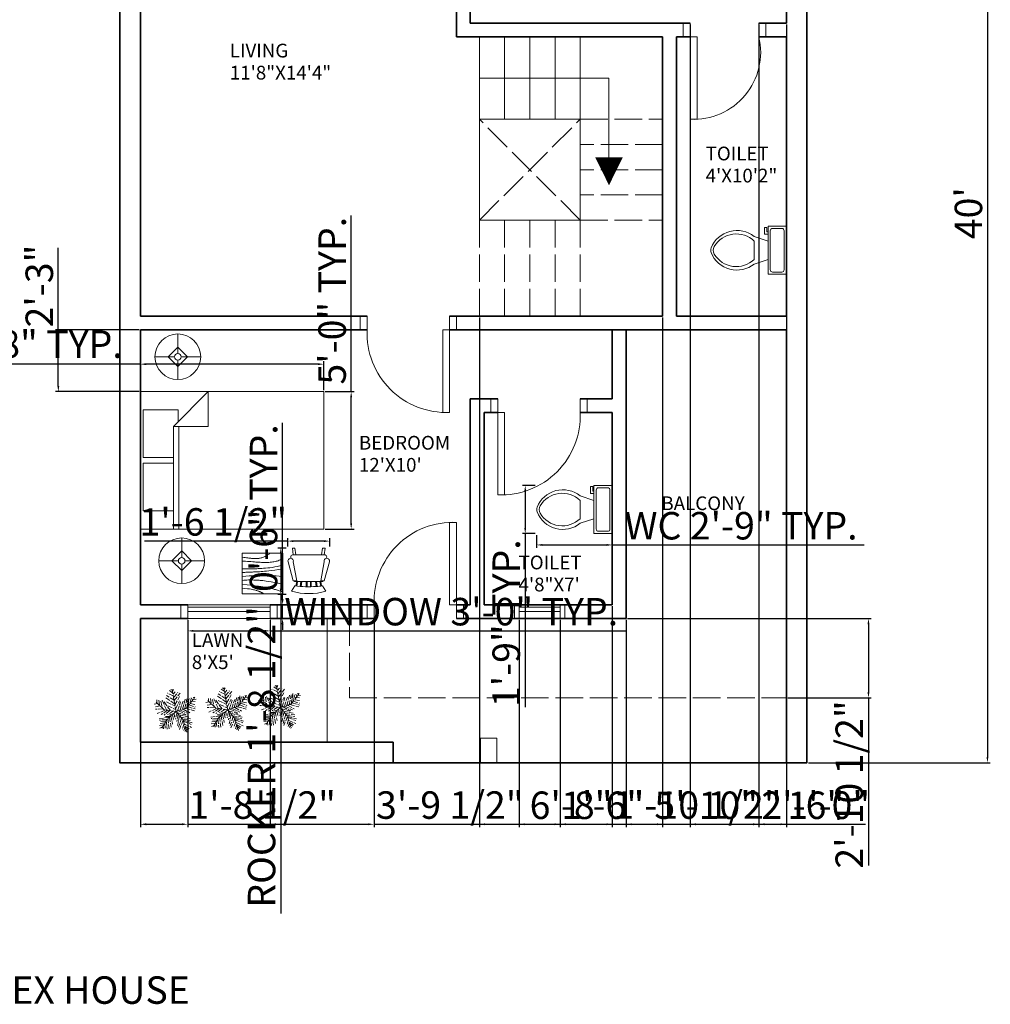
# Model space of a CAD drawing. Units: inches. Extents: x 2446 to 3341, y 462 to 1195.
# Tile 5 of 6: x 2884 to 3308, y 462 to 892. Entities that reach past the tile are written whole.
import ezdxf

# ---------------------------------------------------------------- set-up
doc = ezdxf.new("R2010")
doc.units = ezdxf.units.IN
doc.linetypes.add('ACAD_ISO02W100', pattern=[15, 12, -3])
for name, color, linetype, lineweight in [('A-ANNO-DIMS', 2, 'Continuous', 18), ('A-ANNO-TEXT', 7, 'Continuous', 25), ('A-AREA-IDEN', 7, 'Continuous', 18), ('A-DOOR', 4, 'Continuous', 18), ('A-FLOR-FIXT', 9, 'Continuous', 18), ('A-FLOR-HIDN', 8, 'ACAD_ISO02W100', 18), ('A-FLOR-STRS', 7, 'Continuous', 18), ('A-FLOR-STRS-HIDN', 8, 'ACAD_ISO02W100', 18), ('A-FURN', 8, 'Continuous', 18), ('A-GLAZ', 4, 'Continuous', 18), ('A-WALL', 7, 'Continuous', 35), ('C-PROP', 7, 'Continuous', 35), ('L-PLNT', 3, 'Continuous', 18), ('L-PLNT-BELO', 3, 'ACAD_ISO02W100', 13)]:
    doc.layers.add(name, color=color, linetype=linetype, lineweight=lineweight)
doc.styles.get("Standard").update_dxf_attribs({"font": 'arial.ttf'})
doc.dimstyles.new('ISO-25', dxfattribs={"dimtxt": 12, "dimasz": 2.5, "dimexe": 1.25, "dimexo": 0.625, "dimtad": 1, "dimdec": 1, "dimlunit": 3, "dimtxsty": 'Standard', "dimcen": 2.5, "dimadec": 0, "dimazin": 0, "dimtfac": 1, "dimtdec": 1, "dimtmove": 0, "dimatfit": 3, "dimfxl": 1, "dimarcsym": 0})

# ---------------------------------------------------------------- blocks, each defined once
blk = doc.blocks.new('Toilet - top')
for p, q in [((9.5, -6), (9.5, -2)), ((-10, -8.5), (-8, -8.5)), ((-10, -9.5), (-10, -8.5)), ((-8, -8.5), (-8, -8)), ((-7, -8), (-7, -9.5)), ((-4, -8), (-6, -14)), ((4, -8), (6, -14)), ((-7, -9.5), (-10, -9.5)), ((4, -14), (-4, -14))]:
    blk.add_line(p, q)
blk.add_lwpolyline([(10.5, -8), (10.5, 0), (-10.5, 0), (-10.5, -8)], close=True)
for points in [[(-9.5, -2), (-9.5, -6)], [(8.5, -1), (-8.5, -1)], [(-8.5, -7), (8.5, -7)]]:
    blk.add_lwpolyline(points)
for centre, radius, start, end in [((-8.62, -1.88), 0.884, 81.8699, 188.1301), ((8.62, -1.88), 0.884, 351.8699, 98.1301), ((-8.62, -6.12), 0.884, 171.8699, 278.1301), ((8.62, -6.12), 0.884, 261.8699, 8.1301), ((3.52, -21.58), 12.17, 141.4691, 247.9714), ((4.2, -21.82), 11.33, 136.3677, 238.9468), ((-3.52, -21.58), 12.17, 292.0284, 38.5307), ((-4.2, -21.82), 11.33, 301.053, 43.6321), ((0, -27.88), 4, 245.7318, 294.2682), ((0, -29), 4, 254.8605, 285.1395)]:
    blk.add_arc(centre, radius, start, end)
blk = doc.blocks.new('Bed - Queen')
for p, q in [((0, -80.00003), (0, 0)), ((0, 0), (59.99999, 0)), ((59.99999, 0), (59.99999, -80.00003)), ((7.99999, -1.2), (28.79998, -1.2)), ((7.99999, -14.4), (7.99999, -1.2)), ((28.79998, -1.2), (28.79998, -14.4)), ((31.19999, -1.2), (51.99999, -1.2)), ((31.19999, -14.4), (31.19999, -1.2)), ((51.99999, -1.2), (51.99999, -16.4)), ((0, -14.4), (44.8, -14.4)), ((44.8, -16.8), (0, -16.8)), ((59.99999, -29.6), (44.8, -14.4)), ((44.8, -14.4), (44.8, -29.6)), ((51.99999, -16.4), (46.79936, -16.4)), ((44.8, -29.6), (59.99999, -29.6)), ((59.99999, -80.00003), (0, -80.00003))]:
    blk.add_line(p, q)
blk = doc.blocks.new('Lamp - Table')
for p, q in [((0, 7), (0, 1)), ((-1, 0), (-7, 0)), ((0, 3), (-3, 0)), ((-3, 0), (0, -3)), ((3, 0), (0, 3)), ((0, -3), (3, 0)), ((1, 0), (7, 0)), ((0, -1), (0, -7))]:
    blk.add_line(p, q)
for radius in [7, 1]:
    blk.add_circle((0, 0), radius)
blk = doc.blocks.new('Chair - Rocking')
for p, q in [((-8, -4.5), (-10, -1.5)), ((-7.5, -4.5), (-7, -7)), ((-6.5, -7), (-7.02225, -4.43)), ((-4.5, -7), (-4.96674, -4.19951)), ((-4, -7), (-4.40532, -4.16272)), ((-1.5, -4.05012), (-1.5, -7)), ((-1, -7), (-1, -4.05012)), ((1, -7), (1, -4.04655)), ((1.5, -4.05012), (1.5, -7)), ((4, -7), (4.40187, -4.18694)), ((4.5, -7), (4.96761, -4.19437)), ((6.5, -7), (7, -4.4057)), ((7.5, -4.5), (7, -7)), ((8, -4.5), (10, -1.5)), ((-9, -7.5), (-12, -18.49999)), ((-7, -7.5), (-9, -7.5)), ((-9, -18.49999), (-7, -7.5)), ((-8.23428, -6.99939), (-8.3093, -7.47958)), ((-8.23041, -7), (8.23915, -7)), ((7, -7.5), (9, -7.5)), ((9, -18.49999), (7, -7.5)), ((8.31071, -7.48854), (8.23449, -7.00073)), ((9, -7.5), (12, -18.49999)), ((-10.36644, -20.64523), (-10.5, -21.49999)), ((-9, -22.49999), (-9.5, -26.49999)), ((0, -22.49999), (-9.5, -22.49999)), ((-8, -26.49999), (-7.5, -22.49999)), ((0, -22.49999), (9.5, -22.49999)), ((8, -26.49999), (7.5, -22.49999)), ((9, -22.49999), (9.5, -26.49999)), ((10.5, -21.49999), (10.3575, -20.58798)), ((-9.5, -26.49999), (-8, -26.49999)), ((9.5, -26.49999), (8, -26.49999))]:
    blk.add_line(p, q)
for centre, radius, start, end in [((0, -34.08333), 34.08333, 72.93847, 107.0615), ((0, -68.25004), 64.25, 93.92211, 97.15267), ((0, -68.25004), 64.25, 82.84733, 93.92211), ((-10.5, -18.99999), 1.58114, 161.5651, 18.43495), ((-9.5, -21.49999), 1, 180, 270), ((10.5, -18.99999), 1.58114, 161.5651, 18.43495), ((9.5, -21.49999), 1, 270, 0)]:
    blk.add_arc(centre, radius, start, end)
blk = doc.blocks.new('Table - Square Woodgrain 42 x 42 in.')
blk.add_line((0, -42), (42, -42))
for points in [[(0, -4), (1.704, -4.2172), (3.2358, -4.4188), (4.615, -4.604), (5.8615, -4.7721), (6.9951, -4.9224), (8.0357, -5.0541), (9.0031, -5.1667), (9.9171, -5.2594), (10.7951, -5.3316), (11.6445, -5.3836), (12.4702, -5.4157), (13.277, -5.4283), (14.0698, -5.4217), (14.8535, -5.3964), (15.6331, -5.3526), (16.4133, -5.2908), (17.1986, -5.2103), (17.9913, -5.1062), (18.793, -4.9727), (19.6056, -4.8038), (20.4307, -4.5937), (21.2701, -4.3365), (22.1256, -4.0262), (22.9989, -3.6571), (23.888, -3.2272), (24.7756, -2.7516), (25.6408, -2.2491), (26.4624, -1.7387), (27.2195, -1.2395), (27.891, -0.7703), (28.456, -0.3501), (28.8934, 0.002)], [(0, -42), (0, 0), (42, 0), (42, -42)], [(0, -8), (1.8203, -8.1001), (3.6741, -8.2149), (5.5411, -8.3408), (7.4011, -8.4741), (9.2339, -8.6112), (11.0193, -8.7484), (12.7371, -8.8821), (14.3671, -9.0086), (15.8954, -9.1246), (17.3337, -9.2278), (18.6997, -9.3159), (20.0116, -9.387), (21.2871, -9.4389), (22.5442, -9.4696), (23.8008, -9.477), (25.0749, -9.459), (26.3791, -9.4137), (27.7049, -9.3403), (29.0383, -9.2382), (30.3655, -9.1068), (31.6728, -8.9455), (32.9461, -8.7535), (34.1717, -8.5304), (35.3358, -8.2756), (36.4268, -7.9863), (37.443, -7.6521), (38.3849, -7.2603), (39.253, -6.7986), (40.048, -6.2542), (40.7705, -5.6147), (41.421, -4.8674), (42, -4)], [(42, -12), (39.1784, -12.8621), (36.4519, -13.5654), (33.8246, -14.1294), (31.3004, -14.5731), (28.8832, -14.9161), (26.577, -15.1775), (24.3858, -15.3768), (22.3136, -15.5332), (20.3622, -15.6632), (18.5254, -15.7718), (16.7947, -15.8612), (15.1618, -15.9338), (13.6183, -15.9916), (12.1558, -16.0369), (10.7659, -16.0718), (9.4403, -16.0987), (8.1703, -16.1191), (6.9461, -16.1325), (5.7577, -16.1377), (4.595, -16.1335), (3.4479, -16.1188), (2.3064, -16.0924), (1.1604, -16.0532), (0, -16)], [(42, -16), (37.6529, -16.7365), (33.8802, -17.329), (30.6179, -17.7961), (27.8015, -18.1561), (25.3668, -18.4275), (23.2497, -18.6288), (21.3859, -18.7785), (19.7111, -18.8949), (18.1693, -18.9939), (16.7375, -19.0795), (15.401, -19.1534), (14.1449, -19.217), (12.9544, -19.2717), (11.8148, -19.3191), (10.7113, -19.3606), (9.6291, -19.3976), (8.5534, -19.4323), (7.47, -19.4689), (6.3643, -19.5122), (5.222, -19.5672), (4.0288, -19.6386), (2.7703, -19.7313), (1.4321, -19.8501), (0, -20)], [(0, -24), (3.9243, -23.6805), (7.4766, -23.4138), (10.6891, -23.1954), (13.5943, -23.0205), (16.2247, -22.8847), (18.6125, -22.7832), (20.7903, -22.7116), (22.7903, -22.6651), (24.6563, -22.642), (26.4764, -22.6507), (28.35, -22.7024), (30.3766, -22.8084), (32.6555, -22.98), (35.2861, -23.2283), (38.3678, -23.5645), (42, -24)], [(42, -32), (37.392, -31.017), (33.4585, -30.2231), (30.1291, -29.5949), (27.3334, -29.109), (25.0009, -28.742), (23.0612, -28.4707), (21.4439, -28.2716), (20.0786, -28.1215), (18.8998, -28.0002), (17.8609, -27.9014), (16.9206, -27.8219), (16.0371, -27.7588), (15.1691, -27.709), (14.2748, -27.6693), (13.3128, -27.6368), (12.2415, -27.6083), (11.0295, -27.5824), (9.6867, -27.5643), (8.233, -27.5608), (6.6884, -27.5787), (5.0728, -27.6248), (3.4062, -27.7058), (1.7086, -27.8286), (0, -28)], [(0, -32), (5.4026, -32.5358), (9.9494, -33.019), (13.7424, -33.4553), (16.8834, -33.8505), (19.4743, -34.2106), (21.6171, -34.5413), (23.4136, -34.8486), (24.9657, -35.1382), (26.3614, -35.4156), (27.6332, -35.6841), (28.7995, -35.9467), (29.8788, -36.2064), (30.8897, -36.4661), (31.8507, -36.7288), (32.7802, -36.9973), (33.6968, -37.2747), (34.6175, -37.5635), (35.5531, -37.8651), (36.5128, -38.1805), (37.506, -38.5108), (38.5421, -38.8568), (39.6302, -39.2197), (40.7797, -39.6004), (42, -40)], [(0, -36), (3.0098, -36.2857), (5.5354, -36.5643), (7.6368, -36.8359), (9.374, -37.1009), (10.807, -37.3597), (11.9957, -37.6126), (13.0002, -37.8599), (13.8804, -38.102), (14.6874, -38.3393), (15.4365, -38.5729), (16.1338, -38.8041), (16.7858, -39.0341), (17.3987, -39.264), (17.9787, -39.4952), (18.5322, -39.7288), (19.0655, -39.9662), (19.5832, -40.2081), (20.0842, -40.4544), (20.5657, -40.7046), (21.0249, -40.9581), (21.459, -41.2144), (21.8653, -41.4731), (22.2409, -41.7335), (22.5831, -41.9951)]]:
    blk.add_lwpolyline(points)
blk = doc.blocks.new('*U16')
for p, q in [((-8.737, 47.138), (-17.069, 52.711)), ((-10.186, 53.64), (-13.084, 55.962)), ((0, 0), (-10.5, 57)), ((-9.099, 51.782), (-6.563, 55.962)), ((-31.5, 4.5), (-52.5, 25.5)), ((-48.585, 21.131), (-49.309, 29.026)), ((-43.513, 28.561), (-42.427, 15.558)), ((-38.442, 26.239), (-34.819, 7.663)), ((-35.544, 28.097), (-24.314, 3.947)), ((-14.533, 2.09), (-30.834, 25.31)), ((-3.665, 19.273), (-27.574, 35.527)), ((-5.114, 28.097), (-24.676, 40.636)), ((-7.288, 39.707), (-21.778, 46.673)), ((-7.65, 43.423), (-2.578, 49.46)), ((-5.839, 35.992), (4.667, 48.067)), ((-5.114, 27.632), (10.463, 46.673)), ((-2.941, 16.486), (8.652, 37.85)), ((-1.129, 6.734), (9.014, 26.704)), ((10.101, 3.483), (17.708, 26.239)), ((16.259, 5.805), (23.142, 31.348)), ((22.055, 7.198), (27.489, 32.277)), ((27, 9), (48, 36)), ((27.127, 9.056), (31.112, 35.992)), ((31.836, 30.883), (32.561, 16.486)), ((35.096, 32.741), (37.27, 22.524)), ((38.719, 34.134), (41.979, 28.561)), ((40.53, 25.775), (48.862, 24.846)), ((43.791, 29.954), (51.036, 30.883)), ((44.153, 36.456), (45.239, 32.741)), ((-47.498, 19.737), (-55.83, 18.344)), ((-40.615, 13.7), (-55.105, 10.913)), ((-33.37, 6.269), (-52.207, 5.34)), ((-28.299, 3.483), (-47.86, -5.805)), ((-21.416, 3.018), (-38.079, -8.128)), ((0, 0), (-31.5, 4.5)), ((-15.982, 2.09), (-30.11, -9.521)), ((-24.314, 23.917), (-2.941, 13.7)), ((0, 0), (-22.5, -19.5)), ((-6.563, 1.161), (-21.416, -8.128)), ((-20.691, 13.7), (-1.129, 4.876)), ((0, 0), (27, 9)), ((0, 0), (18, -22.5)), ((3.942, 1.625), (11.187, 24.381)), ((6.478, 1.625), (26.04, -8.592)), ((11.187, 3.483), (30.749, -5.805)), ((18.07, 5.805), (35.096, -3.483)), ((24.229, 7.663), (46.688, 1.625)), ((29.662, 12.307), (48.137, 6.269)), ((33.285, 16.486), (48.862, 10.913)), ((36.183, 19.737), (48.137, 17.88)), ((-17.431, -15.094), (-42.789, -18.809)), ((-24.314, -21.596), (-42.427, -22.06)), ((-22.5, -19.5), (-37.5, -45)), ((-15.257, -12.772), (-30.11, -12.772)), ((-25.038, -23.918), (-22.865, -45.281)), ((-20.691, -18.345), (-17.793, -44.352)), ((-6.563, -5.805), (-19.967, -9.985)), ((-17.069, -15.094), (-12.721, -40.172)), ((-13.446, -11.378), (-8.737, -32.741)), ((-9.461, -8.592), (-6.201, -23.453)), ((-4.752, -3.483), (-3.665, -14.629)), ((2.493, -3.019), (-1.491, -20.202)), ((1.769, -2.555), (24.229, -9.521)), ((5.029, -6.27), (2.131, -25.775)), ((9.014, -11.378), (3.58, -35.992)), ((14.085, -16.951), (6.478, -40.172)), ((7.565, -9.056), (32.198, -14.629)), ((18.07, -22.524), (8.289, -45.745)), ((12.274, -15.094), (36.907, -18.809)), ((16.259, -19.738), (36.183, -22.989)), ((18, -22.5), (27, -52.5)), ((18.433, -22.524), (40.53, -29.026)), ((-28.299, -29.026), (-42.789, -31.348)), ((-30.834, -34.135), (-42.427, -35.528)), ((-34.457, -39.708), (-40.978, -42.494)), ((-26.849, -26.24), (-40.253, -25.775)), ((-32.646, -36.921), (-31.921, -44.352)), ((-29.023, -30.884), (-27.936, -43.887)), ((20.244, -30.419), (15.897, -44.816)), ((19.157, -25.311), (38.719, -33.206)), ((22.78, -37.85), (19.519, -48.532)), ((21.331, -32.741), (39.081, -40.636)), ((22.78, -38.314), (34.372, -44.816)), ((24.591, -45.745), (23.142, -50.854)), ((24.591, -43.423), (30.749, -47.603)), ((26.764, -49.925), (28.213, -50.854))]:
    blk.add_line(p, q)
blk = doc.blocks.new('*D20')
at = {"layer": 'A-ANNO-DIMS', "color": 0, "lineweight": -2, "transparency": 16777216}
for p, q in [((3228.82, 1047.51), (3308.24, 1047.51)), ((3306.99, 1045.01), (3306.99, 570.01)), ((3228.82, 567.51), (3308.24, 567.51))]:
    blk.add_line(p, q, dxfattribs=at)
at = {"layer": 'A-ANNO-DIMS', "color": 0, "transparency": 16777216}
for points in [[(3306.57, 1045.01), (3307.4, 1045.01), (3306.99, 1047.51)], [(3306.57, 570.01), (3307.4, 570.01), (3306.99, 567.51)]]:
    blk.add_solid(points, dxfattribs=at)
at = {"layer": 'Defpoints', "color": 0, "transparency": 16777216}
for p in [(3228.19, 1047.51), (3228.19, 567.51), (3306.99, 567.51)]:
    blk.add_point(p, dxfattribs=at)
at = {"layer": 'A-ANNO-DIMS', "color": 0, "transparency": 16777216, "insert": (3300.24, 807.51), "char_height": 12, "attachment_point": 5, "rotation": 90}
blk.add_mtext("40'", dxfattribs=at)
blk = doc.blocks.new('DOOR-SWING-36IN')
for p, q in [((6, 42), (0, 42)), ((6, 39), (0, 39)), ((6, 3), (0, 3)), ((6, 0), (0, 0))]:
    blk.add_line(p, q)
blk.add_lwpolyline([(6, 3), (42, 3), (42, 6), (6, 6)], close=True)
blk.add_arc((7.5, 4.5), 34.53, 357.5104, 92.4896)
blk = doc.blocks.new('WIN-36IN')
for p, q in [((0, 6), (0, 0)), ((0, 5), (36, 5)), ((36, 0), (36, 6)), ((0, 3), (36, 3))]:
    blk.add_line(p, q)
blk = doc.blocks.new('*D29')
at = {"layer": 'A-ANNO-DIMS', "color": 0, "lineweight": -2, "transparency": 16777216}
for p, q in [((2937.19, 741.58), (2756.92, 741.58)), ((2937.19, 730.2), (2937.19, 742.83)), ((3014.69, 741.58), (2939.69, 741.58)), ((3017.19, 730.2), (3017.19, 742.83))]:
    blk.add_line(p, q, dxfattribs=at)
at = {"layer": 'A-ANNO-DIMS', "color": 0, "transparency": 16777216}
for points in [[(2939.69, 742), (2939.69, 741.16), (2937.19, 741.58)], [(3014.69, 742), (3014.69, 741.16), (3017.19, 741.58)]]:
    blk.add_solid(points, dxfattribs=at)
at = {"layer": 'Defpoints', "color": 0, "transparency": 16777216}
for p in [(2937.19, 741.58), (2937.19, 729.58), (3017.19, 729.58)]:
    blk.add_point(p, dxfattribs=at)
at = {"layer": 'A-ANNO-DIMS', "color": 0, "transparency": 16777216, "insert": (2845.81, 748.78), "char_height": 12, "attachment_point": 5}
blk.add_mtext('QUEEN BED 6\'-8" TYP.', dxfattribs=at)
blk = doc.blocks.new('*D30')
at = {"layer": 'A-ANNO-DIMS', "color": 0, "lineweight": -2, "transparency": 16777216}
for p, q in [((3029.19, 729.58), (3029.19, 806.47)), ((3017.82, 729.58), (3030.44, 729.58)), ((3029.19, 672.08), (3029.19, 727.08)), ((3017.82, 669.58), (3030.44, 669.58))]:
    blk.add_line(p, q, dxfattribs=at)
at = {"layer": 'A-ANNO-DIMS', "color": 0, "transparency": 16777216}
for points in [[(3028.78, 727.08), (3029.61, 727.08), (3029.19, 729.58)], [(3028.78, 672.08), (3029.61, 672.08), (3029.19, 669.58)]]:
    blk.add_solid(points, dxfattribs=at)
at = {"layer": 'Defpoints', "color": 0, "transparency": 16777216}
for p in [(3017.19, 729.58), (3029.19, 729.58), (3017.19, 669.58)]:
    blk.add_point(p, dxfattribs=at)
at = {"layer": 'A-ANNO-DIMS', "color": 0, "transparency": 16777216, "insert": (3022.44, 769.28), "char_height": 12, "attachment_point": 5, "rotation": 90}
blk.add_mtext('5\'-0" TYP.', dxfattribs=at)
blk = doc.blocks.new('*D31')
at = {"layer": 'A-ANNO-DIMS', "color": 0, "lineweight": -2, "transparency": 16777216}
for p, q in [((3110.15, 666.97), (3110.15, 661.39)), ((3143.19, 666.97), (3143.19, 661.39)), ((3112.65, 662.64), (3140.69, 662.64)), ((3143.19, 662.64), (3253.17, 662.64))]:
    blk.add_line(p, q, dxfattribs=at)
at = {"layer": 'A-ANNO-DIMS', "color": 0, "transparency": 16777216}
for points in [[(3112.65, 663.05), (3112.65, 662.22), (3110.15, 662.64)], [(3140.69, 663.05), (3140.69, 662.22), (3143.19, 662.64)]]:
    blk.add_solid(points, dxfattribs=at)
at = {"layer": 'Defpoints', "color": 0, "transparency": 16777216}
for p in [(3110.15, 667.59), (3143.19, 667.59), (3143.19, 662.64)]:
    blk.add_point(p, dxfattribs=at)
at = {"layer": 'A-ANNO-DIMS', "color": 0, "transparency": 16777216, "insert": (3199.43, 669.47), "char_height": 12, "attachment_point": 5}
blk.add_mtext('WC 2\'-9" TYP.', dxfattribs=at)
blk = doc.blocks.new('*D32')
at = {"layer": 'A-ANNO-DIMS', "color": 0, "lineweight": -2, "transparency": 16777216}
for p, q in [((3109.52, 688.59), (3103.94, 688.59)), ((3105.19, 686.09), (3105.19, 670.09)), ((3109.52, 667.59), (3103.94, 667.59)), ((3105.19, 667.59), (3105.19, 591.83))]:
    blk.add_line(p, q, dxfattribs=at)
at = {"layer": 'A-ANNO-DIMS', "color": 0, "transparency": 16777216}
for points in [[(3104.77, 686.09), (3105.61, 686.09), (3105.19, 688.59)], [(3104.77, 670.09), (3105.61, 670.09), (3105.19, 667.59)]]:
    blk.add_solid(points, dxfattribs=at)
at = {"layer": 'Defpoints', "color": 0, "transparency": 16777216}
for p in [(3110.15, 688.59), (3105.19, 667.59), (3110.15, 667.59)]:
    blk.add_point(p, dxfattribs=at)
at = {"layer": 'A-ANNO-DIMS', "color": 0, "transparency": 16777216, "insert": (3098.44, 628.46), "char_height": 12, "attachment_point": 5, "rotation": 90}
blk.add_mtext('1\'-9" TYP.', dxfattribs=at)
blk = doc.blocks.new('*D35')
at = {"layer": 'A-ANNO-DIMS', "color": 0, "lineweight": -2, "transparency": 16777216}
for p, q in [((3000.87, 661.27), (2997.2, 661.27)), ((2998.45, 658.77), (2998.45, 643.5)), ((3000.87, 641), (2997.2, 641)), ((2998.45, 641), (2998.45, 501.63))]:
    blk.add_line(p, q, dxfattribs=at)
at = {"layer": 'A-ANNO-DIMS', "color": 0, "transparency": 16777216}
for points in [[(2998.03, 658.77), (2998.87, 658.77), (2998.45, 661.27)], [(2998.03, 643.5), (2998.87, 643.5), (2998.45, 641)]]:
    blk.add_solid(points, dxfattribs=at)
at = {"layer": 'Defpoints', "color": 0, "transparency": 16777216}
for p in [(3001.49, 661.27), (2998.45, 641), (3001.49, 641)]:
    blk.add_point(p, dxfattribs=at)
at = {"layer": 'A-ANNO-DIMS', "color": 0, "transparency": 16777216, "insert": (2991.62, 570.06), "char_height": 12, "attachment_point": 5, "rotation": 90}
blk.add_mtext('ROCKER 1\'-8 1/2"', dxfattribs=at)
blk = doc.blocks.new('*D36')
at = {"layer": 'A-ANNO-DIMS', "color": 0, "lineweight": -2, "transparency": 16777216}
for p, q in [((3001.49, 664.31), (2939.01, 664.31)), ((3001.49, 661.89), (3001.49, 665.56)), ((3017.33, 664.31), (3003.99, 664.31)), ((3019.83, 661.89), (3019.83, 665.56))]:
    blk.add_line(p, q, dxfattribs=at)
at = {"layer": 'A-ANNO-DIMS', "color": 0, "transparency": 16777216}
for points in [[(3003.99, 664.72), (3003.99, 663.89), (3001.49, 664.31)], [(3017.33, 664.72), (3017.33, 663.89), (3019.83, 664.31)]]:
    blk.add_solid(points, dxfattribs=at)
at = {"layer": 'Defpoints', "color": 0, "transparency": 16777216}
for p in [(3001.49, 664.31), (3001.49, 661.27), (3019.83, 661.27)]:
    blk.add_point(p, dxfattribs=at)
at = {"layer": 'A-ANNO-DIMS', "color": 0, "transparency": 16777216, "insert": (2969, 671.14), "char_height": 12, "attachment_point": 5}
blk.add_mtext('1\'-6 1/2"', dxfattribs=at)
blk = doc.blocks.new('*D49')
at = {"layer": 'A-ANNO-DIMS', "color": 0, "lineweight": -2, "transparency": 16777216}
for p, q in [((2957.84, 629.89), (2957.84, 623.86)), ((2993.84, 629.89), (2993.84, 623.86)), ((2960.34, 625.11), (2991.34, 625.11)), ((2993.84, 625.11), (3149.44, 625.11))]:
    blk.add_line(p, q, dxfattribs=at)
at = {"layer": 'A-ANNO-DIMS', "color": 0, "transparency": 16777216}
for points in [[(2960.34, 625.53), (2960.34, 624.69), (2957.84, 625.11)], [(2991.34, 625.53), (2991.34, 624.69), (2993.84, 625.11)]]:
    blk.add_solid(points, dxfattribs=at)
at = {"layer": 'Defpoints', "color": 0, "transparency": 16777216}
for p in [(2957.84, 630.51), (2993.84, 630.51), (2993.84, 625.11)]:
    blk.add_point(p, dxfattribs=at)
at = {"layer": 'A-ANNO-DIMS', "color": 0, "transparency": 16777216, "insert": (3072.89, 631.95), "char_height": 12, "attachment_point": 5}
blk.add_mtext('WINDOW 3\'-0" TYP.', dxfattribs=at)
blk = doc.blocks.new('*D50')
at = {"layer": 'A-ANNO-DIMS', "color": 0, "lineweight": -2, "transparency": 16777216}
for p, q in [((2999.24, 639.01), (2999.24, 715.91)), ((2994.47, 636.51), (3000.49, 636.51)), ((2999.24, 630.51), (2999.24, 636.51)), ((2994.47, 630.51), (3000.49, 630.51)), ((2999.24, 628.01), (2999.24, 625.51))]:
    blk.add_line(p, q, dxfattribs=at)
at = {"layer": 'A-ANNO-DIMS', "color": 0, "transparency": 16777216}
for points in [[(2998.83, 639.01), (2999.66, 639.01), (2999.24, 636.51)], [(2998.83, 628.01), (2999.66, 628.01), (2999.24, 630.51)]]:
    blk.add_solid(points, dxfattribs=at)
at = {"layer": 'Defpoints', "color": 0, "transparency": 16777216}
for p in [(2993.84, 636.51), (2999.24, 636.51), (2993.84, 630.51)]:
    blk.add_point(p, dxfattribs=at)
at = {"layer": 'A-ANNO-DIMS', "color": 0, "transparency": 16777216, "insert": (2992.49, 678.71), "char_height": 12, "attachment_point": 5, "rotation": 90}
blk.add_mtext('0\'-6" TYP.', dxfattribs=at)
blk = doc.blocks.new('*D61')
at = {"layer": 'A-ANNO-DIMS', "color": 0, "lineweight": -2, "transparency": 16777216}
for p, q in [((3085.19, 761.89), (3085.19, 539.41)), ((3165.19, 761.89), (3165.19, 539.41)), ((3087.69, 540.66), (3162.69, 540.66))]:
    blk.add_line(p, q, dxfattribs=at)
at = {"layer": 'A-ANNO-DIMS', "color": 0, "transparency": 16777216}
for points in [[(3087.69, 541.08), (3087.69, 540.24), (3085.19, 540.66)], [(3162.69, 541.08), (3162.69, 540.24), (3165.19, 540.66)]]:
    blk.add_solid(points, dxfattribs=at)
at = {"layer": 'Defpoints', "color": 0, "transparency": 16777216}
for p in [(3085.19, 762.51), (3165.19, 762.51), (3165.19, 540.66)]:
    blk.add_point(p, dxfattribs=at)
at = {"layer": 'A-ANNO-DIMS', "color": 0, "transparency": 16777216, "insert": (3125.19, 547.41), "char_height": 12, "attachment_point": 5}
blk.add_mtext('6\'-8"', dxfattribs=at)
blk = doc.blocks.new('*D65')
at = {"layer": 'A-ANNO-DIMS', "color": 0, "lineweight": -2, "transparency": 16777216}
for p, q in [((3149.19, 629.89), (3149.19, 539.41)), ((3219.19, 595.22), (3219.19, 539.41)), ((3151.69, 540.66), (3216.69, 540.66))]:
    blk.add_line(p, q, dxfattribs=at)
at = {"layer": 'A-ANNO-DIMS', "color": 0, "transparency": 16777216}
for points in [[(3151.69, 541.08), (3151.69, 540.24), (3149.19, 540.66)], [(3216.69, 541.08), (3216.69, 540.24), (3219.19, 540.66)]]:
    blk.add_solid(points, dxfattribs=at)
at = {"layer": 'Defpoints', "color": 0, "transparency": 16777216}
for p in [(3149.19, 630.51), (3219.19, 595.85), (3219.19, 540.66)]:
    blk.add_point(p, dxfattribs=at)
at = {"layer": 'A-ANNO-DIMS', "color": 0, "transparency": 16777216, "insert": (3184.19, 547.41), "char_height": 12, "attachment_point": 5}
blk.add_mtext('5\'-10"', dxfattribs=at)
blk = doc.blocks.new('*D66')
at = {"layer": 'A-ANNO-DIMS', "color": 0, "lineweight": -2, "transparency": 16777216}
for p, q in [((3149.82, 630.51), (3256.29, 630.51)), ((3255.04, 628.01), (3255.04, 598.35)), ((3219.82, 595.85), (3256.29, 595.85)), ((3255.04, 595.85), (3255.04, 522.71))]:
    blk.add_line(p, q, dxfattribs=at)
at = {"layer": 'A-ANNO-DIMS', "color": 0, "transparency": 16777216}
for points in [[(3254.63, 628.01), (3255.46, 628.01), (3255.04, 630.51)], [(3254.63, 598.35), (3255.46, 598.35), (3255.04, 595.85)]]:
    blk.add_solid(points, dxfattribs=at)
at = {"layer": 'Defpoints', "color": 0, "transparency": 16777216}
for p in [(3149.19, 630.51), (3219.19, 595.85), (3255.04, 595.85)]:
    blk.add_point(p, dxfattribs=at)
at = {"layer": 'A-ANNO-DIMS', "color": 0, "transparency": 16777216, "insert": (3248.21, 558.03), "char_height": 12, "attachment_point": 5, "rotation": 90}
blk.add_mtext('2\'-10 1/2"', dxfattribs=at)
blk = doc.blocks.new('*D69')
at = {"layer": 'A-ANNO-DIMS', "color": 0, "lineweight": -2, "transparency": 16777216}
for p, q in [((3102.48, 629.89), (3102.48, 539.41)), ((3120.48, 629.89), (3120.48, 539.41)), ((3104.98, 540.66), (3117.98, 540.66)), ((3120.48, 540.66), (3155, 540.66))]:
    blk.add_line(p, q, dxfattribs=at)
at = {"layer": 'A-ANNO-DIMS', "color": 0, "transparency": 16777216}
for points in [[(3104.98, 541.08), (3104.98, 540.24), (3102.48, 540.66)], [(3117.98, 541.08), (3117.98, 540.24), (3120.48, 540.66)]]:
    blk.add_solid(points, dxfattribs=at)
at = {"layer": 'Defpoints', "color": 0, "transparency": 16777216}
for p in [(3102.48, 630.51), (3120.48, 630.51), (3120.48, 540.66)]:
    blk.add_point(p, dxfattribs=at)
at = {"layer": 'A-ANNO-DIMS', "color": 0, "transparency": 16777216, "insert": (3138.99, 547.41), "char_height": 12, "attachment_point": 5}
blk.add_mtext('1\'-6"', dxfattribs=at)
blk = doc.blocks.new('*D70')
at = {"layer": 'A-ANNO-DIMS', "color": 0, "lineweight": -2, "transparency": 16777216}
for p, q in [((3143.19, 635.89), (3143.19, 539.41)), ((3120.48, 629.89), (3120.48, 539.41)), ((3122.98, 540.66), (3140.69, 540.66)), ((3143.19, 540.66), (3215, 540.66))]:
    blk.add_line(p, q, dxfattribs=at)
at = {"layer": 'A-ANNO-DIMS', "color": 0, "transparency": 16777216}
for points in [[(3122.98, 541.08), (3122.98, 540.24), (3120.48, 540.66)], [(3140.69, 541.08), (3140.69, 540.24), (3143.19, 540.66)]]:
    blk.add_solid(points, dxfattribs=at)
at = {"layer": 'Defpoints', "color": 0, "transparency": 16777216}
for p in [(3143.19, 636.51), (3120.48, 630.51), (3143.19, 540.66)]:
    blk.add_point(p, dxfattribs=at)
at = {"layer": 'A-ANNO-DIMS', "color": 0, "transparency": 16777216, "insert": (3180.35, 547.49), "char_height": 12, "attachment_point": 5}
blk.add_mtext('1\'-10 1/2"', dxfattribs=at)
blk = doc.blocks.new('*D79')
at = {"layer": 'A-ANNO-DIMS', "color": 0, "lineweight": -2, "transparency": 16777216}
for p, q in [((3177.19, 889.89), (3177.19, 539.41)), ((3207.19, 889.89), (3207.19, 539.41)), ((3179.69, 540.66), (3204.69, 540.66)), ((3207.19, 540.66), (3243.05, 540.66))]:
    blk.add_line(p, q, dxfattribs=at)
at = {"layer": 'A-ANNO-DIMS', "color": 0, "transparency": 16777216}
for points in [[(3179.69, 541.08), (3179.69, 540.24), (3177.19, 540.66)], [(3204.69, 541.08), (3204.69, 540.24), (3207.19, 540.66)]]:
    blk.add_solid(points, dxfattribs=at)
at = {"layer": 'Defpoints', "color": 0, "transparency": 16777216}
for p in [(3177.19, 890.51), (3207.19, 890.51), (3207.19, 540.66)]:
    blk.add_point(p, dxfattribs=at)
at = {"layer": 'A-ANNO-DIMS', "color": 0, "transparency": 16777216, "insert": (3226.37, 547.41), "char_height": 12, "attachment_point": 5}
blk.add_mtext('2\'-6"', dxfattribs=at)
blk = doc.blocks.new('*D80')
at = {"layer": 'A-ANNO-DIMS', "color": 0, "lineweight": -2, "transparency": 16777216}
for p, q in [((3207.19, 889.89), (3207.19, 539.41)), ((3219.19, 889.89), (3219.19, 539.41)), ((3209.69, 540.66), (3216.69, 540.66)), ((3219.19, 540.66), (3253.71, 540.66))]:
    blk.add_line(p, q, dxfattribs=at)
at = {"layer": 'A-ANNO-DIMS', "color": 0, "transparency": 16777216}
for points in [[(3209.69, 541.08), (3209.69, 540.24), (3207.19, 540.66)], [(3216.69, 541.08), (3216.69, 540.24), (3219.19, 540.66)]]:
    blk.add_solid(points, dxfattribs=at)
at = {"layer": 'Defpoints', "color": 0, "transparency": 16777216}
for p in [(3207.19, 890.51), (3219.19, 890.51), (3219.19, 540.66)]:
    blk.add_point(p, dxfattribs=at)
at = {"layer": 'A-ANNO-DIMS', "color": 0, "transparency": 16777216, "insert": (3237.7, 547.41), "char_height": 12, "attachment_point": 5}
blk.add_mtext('1\'-0"', dxfattribs=at)
blk = doc.blocks.new('*D81')
at = {"layer": 'A-ANNO-DIMS', "color": 0, "lineweight": -2, "transparency": 16777216}
for p, q in [((2937.19, 629.89), (2937.19, 539.41)), ((2957.84, 629.89), (2957.84, 539.41)), ((2939.69, 540.66), (2955.34, 540.66)), ((2957.84, 540.66), (3020.32, 540.66))]:
    blk.add_line(p, q, dxfattribs=at)
at = {"layer": 'A-ANNO-DIMS', "color": 0, "transparency": 16777216}
for points in [[(2939.69, 541.08), (2939.69, 540.24), (2937.19, 540.66)], [(2955.34, 541.08), (2955.34, 540.24), (2957.84, 540.66)]]:
    blk.add_solid(points, dxfattribs=at)
at = {"layer": 'Defpoints', "color": 0, "transparency": 16777216}
for p in [(2937.19, 630.51), (2957.84, 630.51), (2957.84, 540.66)]:
    blk.add_point(p, dxfattribs=at)
at = {"layer": 'A-ANNO-DIMS', "color": 0, "transparency": 16777216, "insert": (2990.33, 547.49), "char_height": 12, "attachment_point": 5}
blk.add_mtext('1\'-8 1/2"', dxfattribs=at)
blk = doc.blocks.new('*D82')
at = {"layer": 'A-ANNO-DIMS', "color": 0, "lineweight": -2, "transparency": 16777216}
for p, q in [((2993.84, 629.89), (2993.84, 539.41)), ((3039.19, 629.89), (3039.19, 539.41)), ((2996.34, 540.66), (3036.69, 540.66)), ((3039.19, 540.66), (3102.8, 540.66))]:
    blk.add_line(p, q, dxfattribs=at)
at = {"layer": 'A-ANNO-DIMS', "color": 0, "transparency": 16777216}
for points in [[(2996.34, 541.08), (2996.34, 540.24), (2993.84, 540.66)], [(3036.69, 541.08), (3036.69, 540.24), (3039.19, 540.66)]]:
    blk.add_solid(points, dxfattribs=at)
at = {"layer": 'Defpoints', "color": 0, "transparency": 16777216}
for p in [(2993.84, 630.51), (3039.19, 630.51), (3039.19, 540.66)]:
    blk.add_point(p, dxfattribs=at)
at = {"layer": 'A-ANNO-DIMS', "color": 0, "transparency": 16777216, "insert": (3072.25, 547.49), "char_height": 12, "attachment_point": 5}
blk.add_mtext('3\'-9 1/2"', dxfattribs=at)
blk = doc.blocks.new('*D83')
at = {"layer": 'A-ANNO-DIMS', "color": 0, "lineweight": -2, "transparency": 16777216}
for p, q in [((2901.34, 756.51), (2901.34, 792.36)), ((2936.57, 756.51), (2900.09, 756.51)), ((2901.34, 732.08), (2901.34, 754.01)), ((2936.57, 729.58), (2900.09, 729.58))]:
    blk.add_line(p, q, dxfattribs=at)
at = {"layer": 'A-ANNO-DIMS', "color": 0, "transparency": 16777216}
for points in [[(2900.93, 754.01), (2901.76, 754.01), (2901.34, 756.51)], [(2900.93, 732.08), (2901.76, 732.08), (2901.34, 729.58)]]:
    blk.add_solid(points, dxfattribs=at)
at = {"layer": 'Defpoints', "color": 0, "transparency": 16777216}
for p in [(2901.34, 756.51), (2937.19, 756.51), (2937.19, 729.58)]:
    blk.add_point(p, dxfattribs=at)
at = {"layer": 'A-ANNO-DIMS', "color": 0, "transparency": 16777216, "insert": (2894.59, 775.69), "char_height": 12, "attachment_point": 5, "rotation": 90}
blk.add_mtext('2\'-3"', dxfattribs=at)

msp = doc.modelspace()

# ---------------------------------------------------------------- linework, layer by layer
at = {"layer": 'A-DOOR'}
for p, q in [((3174.19, 884.51), (3174.19, 890.51)), ((3177.19, 884.51), (3177.19, 890.51)), ((3207.19, 884.51), (3207.19, 890.51)), ((3210.19, 884.51), (3210.19, 890.51))]:
    msp.add_line(p, q, dxfattribs=at)
msp.add_lwpolyline([(3177.19, 884.51), (3180.19, 884.51), (3180.19, 848.51), (3177.19, 848.51)], close=True, dxfattribs=at)
msp.add_arc((3178.69, 877.76), 29.29, 267.0643, 13.3245, dxfattribs=at)
at = {"layer": 'A-FLOR-HIDN'}
for p, q in [((3028.41, 630.51), (3028.41, 595.85)), ((3028.41, 595.85), (3219.19, 595.85)), ((3085.7, 567.51), (3085.7, 578.2)), ((3085.7, 578.2), (3092.77, 578.2)), ((3092.77, 578.2), (3092.77, 567.51))]:
    msp.add_line(p, q, dxfattribs=at)
at = {"layer": 'A-FLOR-STRS'}
for p, q in [((3085.19, 848.51), (3085.19, 884.51)), ((3096.19, 848.51), (3096.19, 884.51)), ((3107.19, 848.51), (3107.19, 884.51)), ((3118.19, 848.51), (3118.19, 884.51)), ((3129.19, 804.51), (3129.19, 884.51)), ((3129.19, 848.51), (3085.19, 848.51)), ((3085.19, 804.51), (3085.19, 848.51)), ((3129.19, 804.51), (3085.19, 804.51))]:
    msp.add_line(p, q, dxfattribs=at)
msp.add_lwpolyline([(3085.19, 866.51), (3141.76, 866.51), (3141.76, 831.85)], dxfattribs=at)
msp.add_lwpolyline([(3141.76, 831.85, 12, 0, 0), (3141.76, 819.72, 0, 0, 0)], format="xyseb", dxfattribs=at)
at = {"layer": 'A-FLOR-STRS-HIDN'}
for p, q in [((3129.19, 804.51), (3085.19, 848.51)), ((3085.19, 804.51), (3129.19, 848.51)), ((3129.19, 848.51), (3165.19, 848.51)), ((3165.19, 837.51), (3129.19, 837.51)), ((3165.19, 826.51), (3129.19, 826.51)), ((3165.19, 815.51), (3129.19, 815.51)), ((3085.19, 762.51), (3085.19, 804.51)), ((3096.19, 762.51), (3096.19, 804.51)), ((3107.19, 762.51), (3107.19, 804.51)), ((3118.19, 762.51), (3118.19, 804.51)), ((3129.19, 804.51), (3165.19, 804.51)), ((3129.19, 804.51), (3129.19, 762.51))]:
    msp.add_line(p, q, dxfattribs=at)
at = {"layer": 'A-GLAZ'}
for p, q in [((2954.84, 636.51), (2954.84, 630.51)), ((2957.84, 636.51), (2993.84, 636.51)), ((2996.84, 636.51), (2996.84, 630.51)), ((3100.48, 636.51), (3100.48, 630.51)), ((3120.48, 636.51), (3102.48, 636.51)), ((3102.48, 636.51), (3102.48, 630.51)), ((3102.48, 636.51), (3120.48, 636.51)), ((3120.48, 630.51), (3120.48, 636.51)), ((3122.48, 630.51), (3122.48, 636.51)), ((3102.48, 635.51), (3120.48, 635.51)), ((3102.48, 633.51), (3120.48, 633.51)), ((2957.84, 630.51), (2993.84, 630.51)), ((3102.48, 630.51), (3120.48, 630.51))]:
    msp.add_line(p, q, dxfattribs=at)
at = {"layer": 'A-WALL'}
for p, q in [((3219.19, 890.51), (3219.19, 1038.51)), ((2937.19, 976.51), (2937.19, 762.51)), ((3075.19, 884.51), (3075.19, 896.51)), ((3081.19, 890.51), (3081.19, 896.51)), ((3177.19, 890.51), (3081.19, 890.51)), ((3219.19, 890.51), (3207.19, 890.51)), ((3165.19, 884.51), (3075.19, 884.51)), ((3165.19, 762.51), (3165.19, 884.51)), ((3171.19, 762.51), (3171.19, 884.51)), ((3171.19, 884.51), (3174.19, 884.51)), ((3177.19, 884.51), (3171.19, 884.51)), ((3219.19, 884.51), (3207.19, 884.51)), ((3219.19, 762.51), (3219.19, 884.51)), ((3036.19, 762.51), (2937.19, 762.51)), ((3165.19, 762.51), (3072.19, 762.51)), ((3219.19, 762.51), (3171.19, 762.51)), ((2937.19, 756.51), (2937.19, 636.51)), ((3036.19, 756.51), (2937.19, 756.51)), ((3219.19, 756.51), (3072.19, 756.51)), ((3143.19, 756.51), (3143.19, 726.51)), ((3149.19, 756.51), (3149.19, 630.51)), ((3219.19, 576.51), (3219.19, 756.51)), ((3081.19, 726.51), (3081.19, 636.51)), ((3093.19, 726.51), (3081.19, 726.51)), ((3143.19, 726.51), (3129.19, 726.51)), ((3087.19, 720.51), (3087.19, 636.51)), ((3093.19, 720.51), (3087.19, 720.51)), ((3143.19, 720.51), (3129.19, 720.51)), ((3143.19, 720.51), (3143.19, 636.51)), ((2957.84, 636.51), (2937.19, 636.51)), ((3039.19, 636.51), (2993.84, 636.51)), ((3081.19, 636.51), (3075.19, 636.51)), ((3143.19, 636.51), (3087.19, 636.51)), ((2937.19, 630.51), (2937.19, 576.51)), ((2957.84, 630.51), (2937.19, 630.51)), ((3039.19, 630.51), (2993.84, 630.51)), ((3149.19, 630.51), (3075.19, 630.51)), ((2937.19, 576.51), (3047.47, 576.51)), ((3047.47, 576.51), (3047.47, 567.51)), ((3219.19, 576.51), (3219.19, 567.51))]:
    msp.add_line(p, q, dxfattribs=at)
at = {"layer": 'C-PROP'}
msp.add_lwpolyline([(3219.19, 567.51), (3228.19, 567.51), (3228.19, 1047.51), (2928.19, 1047.51), (2928.19, 567.51), (3219.19, 567.51)], dxfattribs=at)
at = {"layer": 'L-PLNT'}
msp.add_line((3018.73, 630.51), (3018.73, 576.51), dxfattribs=at)

# ---------------------------------------------------------------- block references
at = {"layer": 'A-DOOR', "extrusion": (0, 0, -1), "zscale": -1, "rotation": 269.9999999999981}
msp.add_blockref('DOOR-SWING-36IN', (-3075.19, 762.51), dxfattribs=at)
at = {"layer": 'A-DOOR'}
for p, rotation in [((3090.19, 726.51), 270.0000000000001), ((3078.19, 630.51), 89.99999999999945)]:
    msp.add_blockref('DOOR-SWING-36IN', p, dxfattribs=dict(at, rotation=rotation))
at = {"layer": 'A-FLOR-FIXT', "rotation": 270}
for p in [(3219.19, 791.32), (3143.19, 678.09)]:
    msp.add_blockref('Toilet - top', p, dxfattribs=at)
at = {"layer": 'A-FURN'}
for name, p, xscale, yscale, zscale in [('Lamp - Table', (2953.51, 744.79), 1.425214435139041, 1.425214435139041, 1.425214435139041), ('Lamp - Table', (2955.19, 655.74), 1.425214435139041, 1.425214435139041, 1.425214435139041), ('Table - Square Woodgrain 42 x 42 in.', (2981.54, 658.99), 0.4225793385240015, 0.4225793385240015, 0.4225793385240015)]:
    msp.add_blockref(name, p, dxfattribs=dict(at, xscale=xscale, yscale=yscale, zscale=zscale))
at = {"layer": 'A-FURN', "rotation": 89.99999999999999}
msp.add_blockref('Bed - Queen', (2937.19, 669.58), dxfattribs=at)
at = {"layer": 'A-FURN', "xscale": 0.7507107637491349, "yscale": 0.7507107637491349, "zscale": 0.7507107637491349, "rotation": 180}
msp.add_blockref('Chair - Rocking', (3010.66, 641.37), dxfattribs=at)
at = {"layer": 'A-GLAZ'}
msp.add_blockref('WIN-36IN', (2957.84, 630.51), dxfattribs=at)
at = {"layer": 'L-PLNT-BELO', "xscale": 0.1716127530630565, "yscale": 0.1716127530630565, "zscale": 0.1716127530630565}
for p in [(2952.75, 589.96), (2975.3, 590.67), (2998.32, 591.62)]:
    msp.add_blockref('*U16', p, dxfattribs=at)

# ---------------------------------------------------------------- texts
at = {"layer": 'A-ANNO-TEXT'}
msp.add_text('DUPLEX HOUSE', height=12, dxfattribs=at).set_placement((2838.48, 462.25))
at = {"layer": 'A-AREA-IDEN'}
for s, p in [('LIVING', (2976.21, 875.52)), ('11\'8"X14\'4"', (2976.21, 865.88)), ('TOILET', (3183.95, 830.57)), ('4\'X10\'2"', (3183.95, 820.93)), ('BEDROOM', (3032.57, 704.26)), ("12'X10'", (3032.57, 694.62)), ('BALCONY', (3164.63, 677.83)), ('TOILET', (3102.26, 651.99)), ('4\'8"X7\'', (3102.26, 642.35)), ('LAWN', (2959.61, 618.08)), ("8'X5'", (2959.61, 608.44))]:
    msp.add_text(s, height=6, dxfattribs=at).set_placement(p)

# ---------------------------------------------------------------- dimensions: what is measured, and where the dimension line sits
at = {"layer": 'A-ANNO-DIMS'}
for base, p1, p2, angle, override, picture, middle in [((3306.99, 567.51), (3228.19, 1047.51), (3228.19, 567.51), 90, {"dimclrd": 0, "dimclre": 0, "dimclrt": 0}, '*D20', (3300.24, 807.51)), ((2901.34, 756.51), (2937.19, 729.58), (2937.19, 756.51), 90, {"dimdec": 1, "dimlfac": 1, "dimrnd": 0, "dimzin": 1, "dimdsep": 46, "dimlunit": 4, "dimfrac": 2}, '*D83', (2894.59, 775.69)), ((3001.49, 664.31), (3019.83, 661.27), (3001.49, 661.27), 180, {"dimdec": 1, "dimlfac": 1, "dimrnd": 0, "dimzin": 1, "dimdsep": 46, "dimlunit": 4, "dimfrac": 2}, '*D36', (2969, 671.14)), ((3255.04, 595.85), (3149.19, 630.51), (3219.19, 595.85), 90, {"dimdec": 1, "dimlfac": 1, "dimrnd": 0, "dimzin": 1, "dimdsep": 46, "dimlunit": 4, "dimfrac": 2}, '*D66', (3248.21, 558.03))]:
    dim = msp.add_linear_dim(base=base, p1=p1, p2=p2, angle=angle, dimstyle='ISO-25', override=override, dxfattribs=at)
    dim.commit()
    dim.dimension.update_dxf_attribs({"geometry": picture, "text_midpoint": middle})
for base, p1, p2, picture, middle in [((3207.19, 540.66), (3177.19, 890.51), (3207.19, 890.51), '*D79', (3226.37, 547.41)), ((3219.19, 540.66), (3207.19, 890.51), (3219.19, 890.51), '*D80', (3237.7, 547.41)), ((3165.19, 540.66), (3085.19, 762.51), (3165.19, 762.51), '*D61', (3125.19, 547.41)), ((3143.19, 540.66), (3120.48, 630.51), (3143.19, 636.51), '*D70', (3180.35, 547.49)), ((2957.8433, 540.6603), (2937.1944, 630.5103), (2957.8433, 630.5103), '*D81', (2990.3339, 547.4899)), ((3039.1944, 540.6603), (2993.8433, 630.5103), (3039.1944, 630.5103), '*D82', (3072.2458, 547.494)), ((3120.48, 540.66), (3102.48, 630.51), (3120.48, 630.51), '*D69', (3138.99, 547.41)), ((3219.19, 540.66), (3149.19, 630.51), (3219.19, 595.85), '*D65', (3184.19, 547.41))]:
    dim = msp.add_linear_dim(base=base, p1=p1, p2=p2, dimstyle='ISO-25', override={"dimdec": 1, "dimlfac": 1, "dimrnd": 0, "dimzin": 1, "dimdsep": 46, "dimlunit": 4, "dimfrac": 2}, dxfattribs=at)
    dim.commit()
    dim.dimension.update_dxf_attribs({"geometry": picture, "text_midpoint": middle})
for base, p1, p2, angle, text, picture, middle in [((3029.19, 729.58), (3017.19, 669.58), (3017.19, 729.58), 90, '<> TYP.', '*D30', (3022.44, 769.28)), ((2937.19, 741.58), (3017.19, 729.58), (2937.19, 729.58), 180, 'QUEEN BED <> TYP.', '*D29', (2845.81, 748.78)), ((2999.24, 636.51), (2993.84, 630.51), (2993.84, 636.51), 90, '<> TYP.', '*D50', (2992.49, 678.71)), ((3105.19, 667.59), (3110.15, 688.59), (3110.15, 667.59), 270, '<> TYP.', '*D32', (3098.44, 628.46)), ((2998.45, 641), (3001.49, 661.27), (3001.49, 641), 270, 'ROCKER <>', '*D35', (2991.62, 570.06))]:
    dim = msp.add_linear_dim(base=base, p1=p1, p2=p2, angle=angle, text=text, dimstyle='ISO-25', override={"dimdec": 1, "dimlfac": 1, "dimrnd": 0, "dimzin": 1, "dimdsep": 46, "dimlunit": 4, "dimfrac": 2}, dxfattribs=at)
    dim.commit()
    dim.dimension.update_dxf_attribs({"geometry": picture, "text_midpoint": middle})
for base, p1, p2, text, picture, middle in [((3143.19, 662.64), (3110.15, 667.59), (3143.19, 667.59), 'WC <> TYP.', '*D31', (3199.43, 669.47)), ((2993.84, 625.11), (2957.84, 630.51), (2993.84, 630.51), 'WINDOW <> TYP.', '*D49', (3072.89, 631.95))]:
    dim = msp.add_linear_dim(base=base, p1=p1, p2=p2, text=text, dimstyle='ISO-25', override={"dimdec": 1, "dimlfac": 1, "dimrnd": 0, "dimzin": 1, "dimdsep": 46, "dimlunit": 4, "dimfrac": 2}, dxfattribs=at)
    dim.commit()
    dim.dimension.update_dxf_attribs({"geometry": picture, "text_midpoint": middle})

doc.saveas('drawing.dxf')
